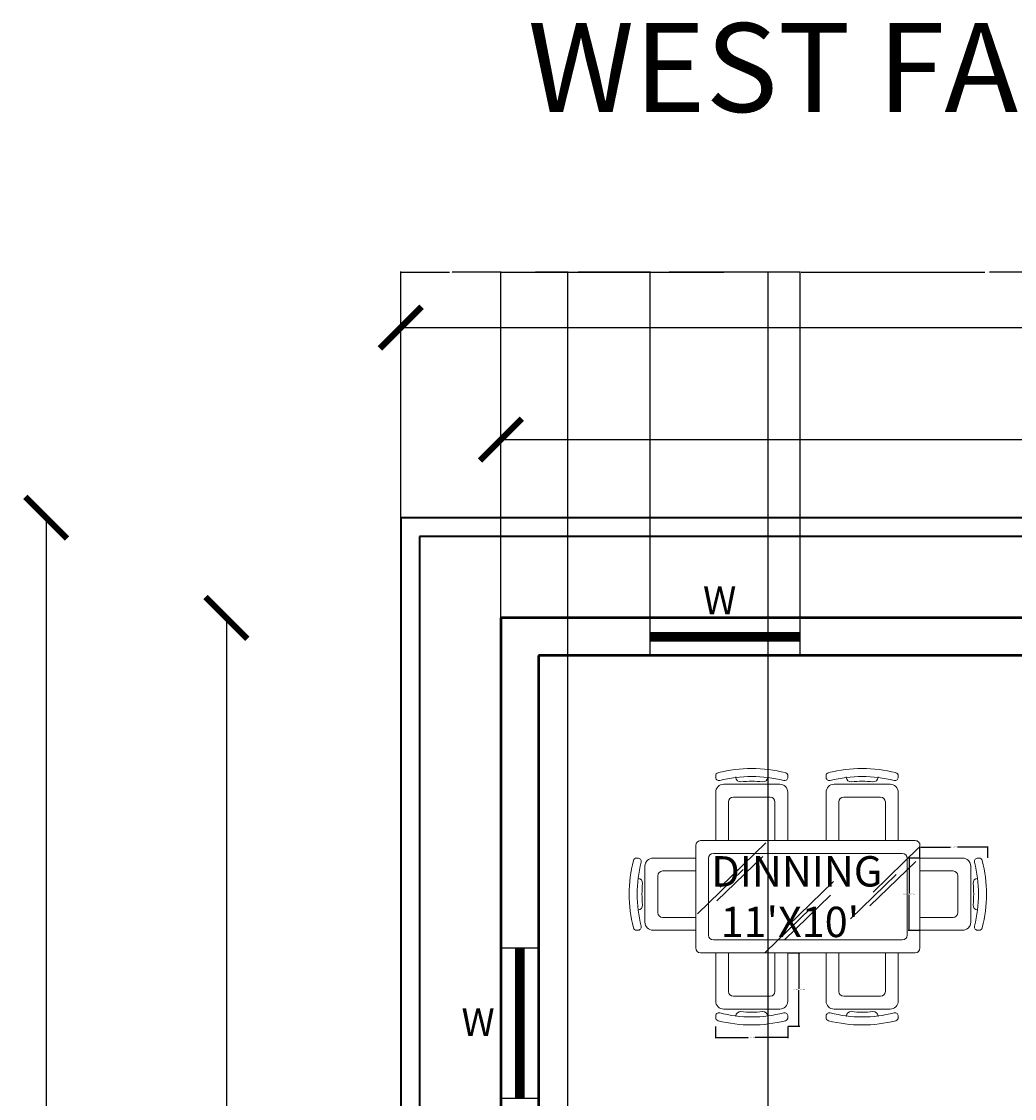
# Model space of a CAD drawing. Units: inches. Extents: x 338 to 1188, y -996 to 127.
# Tile 7 of 15: x 482 to 720, y -131 to 127. Entities that reach past the tile are written whole.
import ezdxf

# ---------------------------------------------------------------- set-up
doc = ezdxf.new("R2010")
doc.units = ezdxf.units.IN
doc.header["$MEASUREMENT"] = 0
for name, color, linetype, lineweight in [('A-ANNO-DIMS', 5, 'Continuous', 18), ('A-ANNO-TEXT', 7, 'Continuous', 18), ('A-ANNO-TITL', 7, 'Continuous', 35), ('A-AREA-IDEN', 8, 'Continuous', 18), ('A-GLAZ-PATT', 5, 'Continuous', 13), ('C-PROP', 1, 'Continuous', 35), ('wall', 1, 'Continuous', 50), ('win', 5, 'Continuous', 25)]:
    doc.layers.add(name, color=color, linetype=linetype, lineweight=lineweight)
doc.layers.add('furniture', color=50, linetype='Continuous', lineweight=13, transparency=0.8)
doc.styles.get("Standard").update_dxf_attribs({"font": 'arial.ttf'})
doc.dimstyles.get("Standard").update_dxf_attribs({"dimtxt": 0.18, "dimasz": 0.18, "dimexe": 0.18, "dimexo": 0.0625, "dimgap": 0.09, "dimtad": 0, "dimtih": 1, "dimtoh": 1, "dimdec": 1, "dimzin": 0, "dimdsep": 46, "dimlunit": 4, "dimtxsty": 'Standard', "dimcen": 0.09, "dimadec": 0, "dimazin": 0, "dimtfac": 1, "dimtdec": 1, "dimtofl": 0, "dimtmove": 0, "dimatfit": 3, "dimfxl": 1, "dimtolj": 1, "dimtzin": 0, "dimarcsym": 0})

# ---------------------------------------------------------------- blocks, each defined once
blk = doc.blocks.new('_ArchTick')
at = {"color": 0, "linetype": 'ByBlock', "const_width": 0.15}
blk.add_lwpolyline([(-0.5, -0.5), (0.5, 0.5)], dxfattribs=at)
blk = doc.blocks.new('*D4')
at = {"layer": 'A-ANNO-DIMS', "color": 0, "lineweight": -2, "transparency": 16777216}
for p, q in [((596.96, 26.99), (765.33, 26.99)), ((956.96, 26.99), (788.6, 26.99))]:
    blk.add_line(p, q, dxfattribs=at)
at = {"layer": 'Defpoints', "color": 0, "transparency": 16777216}
for p in [(956.96, 26.99), (596.96, -15.73), (956.96, -15.73)]:
    blk.add_point(p, dxfattribs=at)
at = {"layer": 'A-ANNO-DIMS', "color": 0, "lineweight": -2, "transparency": 16777216, "xscale": 10, "yscale": 10, "zscale": 10, "rotation": 180}
blk.add_blockref('_ArchTick', (596.96, 26.99), dxfattribs=at)
at = {"layer": 'A-ANNO-DIMS', "color": 0, "lineweight": -2, "transparency": 16777216, "xscale": 10, "yscale": 10, "zscale": 10}
blk.add_blockref('_ArchTick', (956.96, 26.99), dxfattribs=at)
at = {"layer": 'A-ANNO-DIMS', "color": 0, "transparency": 16777216, "insert": (776.96, 26.99), "char_height": 9, "attachment_point": 5}
blk.add_mtext("\\A1;30'", dxfattribs=at)
blk = doc.blocks.new('*D5')
at = {"layer": 'A-ANNO-DIMS', "color": 0, "lineweight": -2, "transparency": 16777216}
for p, q in [((572.96, 53.81), (765.33, 53.81)), ((980.96, 53.81), (788.6, 53.81))]:
    blk.add_line(p, q, dxfattribs=at)
at = {"layer": 'Defpoints', "color": 0, "transparency": 16777216}
for p in [(980.96, 53.81), (572.96, 8.27), (980.96, 8.27)]:
    blk.add_point(p, dxfattribs=at)
at = {"layer": 'A-ANNO-DIMS', "color": 0, "lineweight": -2, "transparency": 16777216, "xscale": 10, "yscale": 10, "zscale": 10, "rotation": 180}
blk.add_blockref('_ArchTick', (572.96, 53.81), dxfattribs=at)
at = {"layer": 'A-ANNO-DIMS', "color": 0, "lineweight": -2, "transparency": 16777216, "xscale": 10, "yscale": 10, "zscale": 10}
blk.add_blockref('_ArchTick', (980.96, 53.81), dxfattribs=at)
at = {"layer": 'A-ANNO-DIMS', "color": 0, "transparency": 16777216, "insert": (776.96, 53.81), "char_height": 9, "attachment_point": 5}
blk.add_mtext("\\A1;34'", dxfattribs=at)
blk = doc.blocks.new('*D6')
at = {"layer": 'A-ANNO-DIMS', "color": 0, "lineweight": -2, "transparency": 16777216}
for p, q in [((531.19, -15.73), (531.19, -304.1)), ((531.19, -615.73), (531.19, -327.37))]:
    blk.add_line(p, q, dxfattribs=at)
at = {"layer": 'Defpoints', "color": 0, "transparency": 16777216}
for p in [(596.96, -15.73), (531.19, -615.73), (596.96, -615.73)]:
    blk.add_point(p, dxfattribs=at)
at = {"layer": 'A-ANNO-DIMS', "color": 0, "lineweight": -2, "transparency": 16777216, "xscale": 10, "yscale": 10, "zscale": 10}
for p, rotation in [((531.19, -15.73), 90), ((531.19, -615.73), 270)]:
    blk.add_blockref('_ArchTick', p, dxfattribs=dict(at, rotation=rotation))
at = {"layer": 'A-ANNO-DIMS', "color": 0, "transparency": 16777216, "insert": (531.19, -315.73), "char_height": 9, "attachment_point": 5, "rotation": 90}
blk.add_mtext("\\A1;50'", dxfattribs=at)
blk = doc.blocks.new('*D7')
at = {"layer": 'A-ANNO-DIMS', "color": 0, "lineweight": -2, "transparency": 16777216}
for p, q in [((488.01, 8.27), (488.01, -388.07)), ((488.01, -807.73), (488.01, -411.39))]:
    blk.add_line(p, q, dxfattribs=at)
at = {"layer": 'Defpoints', "color": 0, "transparency": 16777216}
for p in [(572.96, 8.27), (488.01, -807.73), (572.96, -807.73)]:
    blk.add_point(p, dxfattribs=at)
at = {"layer": 'A-ANNO-DIMS', "color": 0, "lineweight": -2, "transparency": 16777216, "xscale": 10, "yscale": 10, "zscale": 10}
for p, rotation in [((488.01, 8.27), 90), ((488.01, -807.73), 270)]:
    blk.add_blockref('_ArchTick', p, dxfattribs=dict(at, rotation=rotation))
at = {"layer": 'A-ANNO-DIMS', "color": 0, "transparency": 16777216, "insert": (488.01, -399.73), "char_height": 9, "attachment_point": 5, "rotation": 90}
blk.add_mtext("\\A1;68'", dxfattribs=at)
blk = doc.blocks.new('CHAIR-DINING-SIDE')
for p, q in [((6.72, 13.5), (-6.72, 13.5)), ((-3.84, 15.13), (-3.84, 15.25)), ((3.84, 15.13), (3.84, 15.25)), ((-8.63, 11.76), (-8.63, 11.36)), ((-8.63, 11.58), (-8.63, 0)), ((4.41, 10.43), (-4.41, 10.43)), ((8.63, 11.36), (8.63, 11.76)), ((8.63, 0), (8.63, 11.58)), ((-5.56, 9.28), (-5.56, 0)), ((5.56, 0), (5.56, 9.28))]:
    blk.add_line(p, q)
for centre, radius, start, end in [((-7.87, 15.54), 0.768, 104.147, 185.9216), ((0, -15.67), 32.96, 75.853, 104.147), ((7.87, 15.54), 0.768, 354.0784, 75.853), ((-9.78, 15.34), 1.15, 354.0784, 5.9216), ((-7.87, 15.15), 0.768, 174.0784, 284.3214), ((-6.72, 11.58), 1.92, 90, 180), ((0, -15.67), 31.04, 75.6786, 104.3214), ((-2.69, 15.25), 1.15, 186.0281, 274.9654), ((0, -15.67), 29.89, 85.0346, 94.9654), ((2.69, 15.25), 1.15, 265.0346, 353.9719), ((6.72, 11.58), 1.92, 0, 90), ((7.87, 15.15), 0.768, 255.6786, 5.9216), ((9.78, 15.34), 1.15, 174.0784, 185.9216), ((-4.41, 9.28), 1.15, 90, 180), ((4.41, 9.28), 1.15, 0, 90)]:
    blk.add_arc(centre, radius, start, end)
blk = doc.blocks.new('CHAIR-DINING-END')
for p, q in [((-10.42, 8.63), (-10.02, 8.63)), ((-10.24, 8.63), (0, 8.63)), ((-12.16, -6.72), (-12.16, 6.72)), ((-7.94, 5.56), (0, 5.56)), ((-13.79, 3.84), (-13.91, 3.84)), ((-9.09, -4.41), (-9.09, 4.41)), ((-13.79, -3.84), (-13.91, -3.84)), ((0, -5.56), (-7.94, -5.56)), ((-10.02, -8.63), (-10.42, -8.63)), ((0, -8.63), (-10.24, -8.63))]:
    blk.add_line(p, q)
for centre, radius, start, end in [((17.01, 0), 32.96, 165.853, 194.147), ((-14.2, 7.87), 0.768, 84.0784, 165.853), ((-14.01, 9.78), 1.15, 264.0784, 275.9216), ((-13.81, 7.87), 0.768, 345.6786, 95.9216), ((-10.24, 6.72), 1.92, 90, 180), ((17.01, 0), 31.04, 165.6786, 194.3214), ((-7.94, 4.41), 1.15, 90, 180), ((-13.91, 2.69), 1.15, 355.0346, 83.9719), ((17.01, 0), 29.89, 175.0346, 184.9654), ((-13.91, -2.69), 1.15, 276.0281, 4.9654), ((-7.94, -4.41), 1.15, 180, 270), ((-13.81, -7.87), 0.768, 264.0784, 14.3214), ((-10.24, -6.72), 1.92, 180, 270), ((-14.2, -7.87), 0.768, 194.147, 275.9216), ((-14.01, -9.78), 1.15, 84.0784, 95.9216)]:
    blk.add_arc(centre, radius, start, end)
blk = doc.blocks.new('*D15')
at = {"layer": 'A-ANNO-DIMS', "color": 0, "lineweight": -2, "transparency": 16777216}
for p, q in [((665.79, -95.98), (668.55, -95.98)), ((668.37, -96.16), (668.37, -104.6)), ((668.37, -113.42), (668.37, -104.97)), ((665.79, -113.6), (668.55, -113.6))]:
    blk.add_line(p, q, dxfattribs=at)
at = {"layer": 'A-ANNO-DIMS', "color": 0, "transparency": 16777216}
for points in [[(668.34, -96.16), (668.4, -96.16), (668.37, -95.98)], [(668.34, -113.42), (668.4, -113.42), (668.37, -113.6)]]:
    blk.add_solid(points, dxfattribs=at)
at = {"layer": 'Defpoints', "color": 0, "transparency": 16777216}
for p in [(665.73, -95.98), (665.73, -113.6), (668.37, -113.6)]:
    blk.add_point(p, dxfattribs=at)
at = {"layer": 'A-ANNO-DIMS', "color": 0, "transparency": 16777216, "insert": (668.37, -104.79), "char_height": 0.18, "attachment_point": 5}
blk.add_mtext('\\A1;SIDE CHAIR 1\'-5 1/2" TYP.', dxfattribs=at)
blk = doc.blocks.new('*D16')
at = {"layer": 'A-ANNO-DIMS', "color": 0, "lineweight": -2, "transparency": 16777216}
for p, q in [((648.39, -113.66), (648.39, -116.42)), ((665.73, -113.66), (665.73, -116.42)), ((648.57, -116.24), (656.22, -116.24)), ((665.55, -116.24), (657.9, -116.24))]:
    blk.add_line(p, q, dxfattribs=at)
at = {"layer": 'A-ANNO-DIMS', "color": 0, "transparency": 16777216}
for points in [[(648.57, -116.21), (648.57, -116.27), (648.39, -116.24)], [(665.55, -116.21), (665.55, -116.27), (665.73, -116.24)]]:
    blk.add_solid(points, dxfattribs=at)
at = {"layer": 'Defpoints', "color": 0, "transparency": 16777216}
for p in [(648.39, -113.6), (665.73, -113.6), (648.39, -116.24)]:
    blk.add_point(p, dxfattribs=at)
at = {"layer": 'A-ANNO-DIMS', "color": 0, "transparency": 16777216, "insert": (657.06, -116.24), "char_height": 0.18, "attachment_point": 5}
blk.add_mtext('\\A1;1\'-5 1/2" TYP.', dxfattribs=at)
blk = doc.blocks.new('*D17')
at = {"layer": 'A-ANNO-DIMS', "color": 0, "lineweight": -2, "transparency": 16777216}
for p, q in [((697.3, -73.27), (694.58, -73.27)), ((694.76, -73.45), (694.76, -81.76)), ((694.76, -90.43), (694.76, -82.12)), ((697.3, -90.61), (694.58, -90.61))]:
    blk.add_line(p, q, dxfattribs=at)
at = {"layer": 'A-ANNO-DIMS', "color": 0, "transparency": 16777216}
for points in [[(694.73, -73.45), (694.79, -73.45), (694.76, -73.27)], [(694.73, -90.43), (694.79, -90.43), (694.76, -90.61)]]:
    blk.add_solid(points, dxfattribs=at)
at = {"layer": 'Defpoints', "color": 0, "transparency": 16777216}
for p in [(697.36, -73.27), (694.76, -90.61), (697.36, -90.61)]:
    blk.add_point(p, dxfattribs=at)
at = {"layer": 'A-ANNO-DIMS', "color": 0, "transparency": 16777216, "insert": (694.76, -81.94), "char_height": 0.18, "attachment_point": 5}
blk.add_mtext('\\A1;END CHAIR 1\'-5 1/2" TYP.', dxfattribs=at)
blk = doc.blocks.new('*D18')
at = {"layer": 'A-ANNO-DIMS', "color": 0, "lineweight": -2, "transparency": 16777216}
for p, q in [((697.36, -73.21), (697.36, -70.49)), ((697.54, -70.67), (704.67, -70.67)), ((713.47, -70.67), (706.34, -70.67)), ((713.65, -73.21), (713.65, -70.49))]:
    blk.add_line(p, q, dxfattribs=at)
at = {"layer": 'A-ANNO-DIMS', "color": 0, "transparency": 16777216}
for points in [[(697.54, -70.64), (697.54, -70.7), (697.36, -70.67)], [(713.47, -70.64), (713.47, -70.7), (713.65, -70.67)]]:
    blk.add_solid(points, dxfattribs=at)
at = {"layer": 'Defpoints', "color": 0, "transparency": 16777216}
for p in [(697.36, -70.67), (697.36, -73.27), (713.65, -73.27)]:
    blk.add_point(p, dxfattribs=at)
at = {"layer": 'A-ANNO-DIMS', "color": 0, "transparency": 16777216, "insert": (705.51, -70.67), "char_height": 0.18, "attachment_point": 5}
blk.add_mtext('\\A1;1\'-4 1/2" TYP.', dxfattribs=at)
blk = doc.blocks.new('*D24')
at = {"layer": 'A-ANNO-DIMS', "color": 0, "lineweight": -2, "transparency": 16777216}
for p, q in [((572.96, 8.33), (572.96, 67.25)), ((596.96, -15.67), (596.96, 67.25)), ((573.14, 67.07), (584.63, 67.07)), ((596.78, 67.07), (585.29, 67.07))]:
    blk.add_line(p, q, dxfattribs=at)
at = {"layer": 'A-ANNO-DIMS', "color": 0, "transparency": 16777216}
for points in [[(573.14, 67.1), (573.14, 67.04), (572.96, 67.07)], [(596.78, 67.1), (596.78, 67.04), (596.96, 67.07)]]:
    blk.add_solid(points, dxfattribs=at)
at = {"layer": 'Defpoints', "color": 0, "transparency": 16777216}
for p in [(596.96, 67.07), (572.96, 8.27), (596.96, -15.73)]:
    blk.add_point(p, dxfattribs=at)
at = {"layer": 'A-ANNO-DIMS', "color": 0, "transparency": 16777216, "insert": (584.96, 67.07), "char_height": 0.18, "attachment_point": 5}
blk.add_mtext('\\A1;2\'-0"', dxfattribs=at)
blk = doc.blocks.new('*D33')
at = {"layer": 'A-ANNO-DIMS', "color": 0, "lineweight": -2, "transparency": 16777216}
for p, q in [((632.69, -15.67), (632.69, 67.25)), ((668.69, -15.67), (668.69, 67.25)), ((632.87, 67.07), (650.37, 67.07)), ((668.51, 67.07), (651.02, 67.07))]:
    blk.add_line(p, q, dxfattribs=at)
at = {"layer": 'A-ANNO-DIMS', "color": 0, "transparency": 16777216}
for points in [[(632.87, 67.1), (632.87, 67.04), (632.69, 67.07)], [(668.51, 67.1), (668.51, 67.04), (668.69, 67.07)]]:
    blk.add_solid(points, dxfattribs=at)
at = {"layer": 'Defpoints', "color": 0, "transparency": 16777216}
for p in [(668.69, 67.07), (632.69, -15.73), (668.69, -15.73)]:
    blk.add_point(p, dxfattribs=at)
at = {"layer": 'A-ANNO-DIMS', "color": 0, "transparency": 16777216, "insert": (650.69, 67.07), "char_height": 0.18, "attachment_point": 5}
blk.add_mtext('\\A1;3\'-0"', dxfattribs=at)
blk = doc.blocks.new('*D34')
at = {"layer": 'A-ANNO-DIMS', "color": 0, "lineweight": -2, "transparency": 16777216}
for p, q in [((612.96, -615.67), (612.96, 67.25)), ((660.96, -615.67), (660.96, 67.25)), ((613.14, 67.07), (636.63, 67.07)), ((660.78, 67.07), (637.3, 67.07))]:
    blk.add_line(p, q, dxfattribs=at)
at = {"layer": 'A-ANNO-DIMS', "color": 0, "transparency": 16777216}
for points in [[(613.14, 67.1), (613.14, 67.04), (612.96, 67.07)], [(660.78, 67.1), (660.78, 67.04), (660.96, 67.07)]]:
    blk.add_solid(points, dxfattribs=at)
at = {"layer": 'Defpoints', "color": 0, "transparency": 16777216}
for p in [(660.96, 67.07), (612.96, -615.73), (660.96, -615.73)]:
    blk.add_point(p, dxfattribs=at)
at = {"layer": 'A-ANNO-DIMS', "color": 0, "transparency": 16777216, "insert": (636.96, 67.07), "char_height": 0.18, "attachment_point": 5}
blk.add_mtext('\\A1;4\'-0"', dxfattribs=at)
blk = doc.blocks.new('*D48')
at = {"layer": 'A-ANNO-DIMS', "color": 0, "lineweight": -2, "transparency": 16777216}
for p, q in [((596.96, -615.67), (596.96, 67.25)), ((612.96, -615.67), (612.96, 67.25)), ((597.14, 67.07), (604.64, 67.07)), ((612.78, 67.07), (605.28, 67.07))]:
    blk.add_line(p, q, dxfattribs=at)
at = {"layer": 'A-ANNO-DIMS', "color": 0, "transparency": 16777216}
for points in [[(597.14, 67.1), (597.14, 67.04), (596.96, 67.07)], [(612.78, 67.1), (612.78, 67.04), (612.96, 67.07)]]:
    blk.add_solid(points, dxfattribs=at)
at = {"layer": 'Defpoints', "color": 0, "transparency": 16777216}
for p in [(612.96, 67.07), (596.96, -615.73), (612.96, -615.73)]:
    blk.add_point(p, dxfattribs=at)
at = {"layer": 'A-ANNO-DIMS', "color": 0, "transparency": 16777216, "insert": (604.96, 67.07), "char_height": 0.18, "attachment_point": 5}
blk.add_mtext('\\A1;1\'-4"', dxfattribs=at)
blk = doc.blocks.new('*D49')
at = {"layer": 'A-ANNO-DIMS', "color": 0, "lineweight": -2, "transparency": 16777216}
for p, q in [((596.96, -15.67), (596.96, 67.25)), ((632.69, -15.67), (632.69, 67.25)), ((597.14, 67.07), (614.22, 67.07)), ((632.51, 67.07), (615.44, 67.07))]:
    blk.add_line(p, q, dxfattribs=at)
at = {"layer": 'A-ANNO-DIMS', "color": 0, "transparency": 16777216}
for points in [[(597.14, 67.1), (597.14, 67.04), (596.96, 67.07)], [(632.51, 67.1), (632.51, 67.04), (632.69, 67.07)]]:
    blk.add_solid(points, dxfattribs=at)
at = {"layer": 'Defpoints', "color": 0, "transparency": 16777216}
for p in [(632.69, 67.07), (596.96, -15.73), (632.69, -15.73)]:
    blk.add_point(p, dxfattribs=at)
at = {"layer": 'A-ANNO-DIMS', "color": 0, "transparency": 16777216, "insert": (614.83, 67.07), "char_height": 0.18, "attachment_point": 5}
blk.add_mtext('\\A1;2\'-11 1/2"', dxfattribs=at)
blk = doc.blocks.new('*D50')
at = {"layer": 'A-ANNO-DIMS', "color": 0, "lineweight": -2, "transparency": 16777216}
for p, q in [((668.69, -15.67), (668.69, 67.25)), ((758.21, -15.67), (758.21, 67.25)), ((668.87, 67.07), (712.91, 67.07)), ((758.03, 67.07), (713.99, 67.07))]:
    blk.add_line(p, q, dxfattribs=at)
at = {"layer": 'A-ANNO-DIMS', "color": 0, "transparency": 16777216}
for points in [[(668.87, 67.1), (668.87, 67.04), (668.69, 67.07)], [(758.03, 67.1), (758.03, 67.04), (758.21, 67.07)]]:
    blk.add_solid(points, dxfattribs=at)
at = {"layer": 'Defpoints', "color": 0, "transparency": 16777216}
for p in [(758.21, 67.07), (668.69, -15.73), (758.21, -15.73)]:
    blk.add_point(p, dxfattribs=at)
at = {"layer": 'A-ANNO-DIMS', "color": 0, "transparency": 16777216, "insert": (713.45, 67.07), "char_height": 0.18, "attachment_point": 5}
blk.add_mtext('\\A1;7\'-5 1/2"', dxfattribs=at)

msp = doc.modelspace()

# ---------------------------------------------------------------- hatches: boundary and pattern name
at = {"layer": 'A-GLAZ-PATT'}
h = msp.add_hatch(dxfattribs=at)
h.set_pattern_fill('ANSI31', color=256)
h.paths.add_polyline_path([(953.46, -405.07), (951.46, -405.07), (951.46, -429.07), (953.46, -429.07)])
h.paths.add_polyline_path([(953.46, -485.22), (951.46, -485.22), (951.46, -521.22), (953.46, -521.22)])
h.paths.add_polyline_path([(794.21, -19.23), (758.21, -19.23), (758.21, -21.23), (794.21, -21.23)])
h.paths.add_polyline_path([(668.69, -19.23), (632.69, -19.23), (632.69, -21.23), (668.69, -21.23)])
h.paths.add_polyline_path([(602.46, -94.89), (600.46, -94.89), (600.46, -130.89), (602.46, -130.89)])
h.paths.add_polyline_path([(602.46, -243.73), (600.46, -243.73), (600.46, -315.73), (602.46, -315.73)])

# ---------------------------------------------------------------- linework, layer by layer
at = {"layer": 'C-PROP'}
for p, q in [((572.96, 8.27), (572.96, -807.73)), ((980.96, 8.27), (572.96, 8.27)), ((976.46, 3.77), (577.46, 3.77)), ((577.46, 3.77), (577.46, -803.23))]:
    msp.add_line(p, q, dxfattribs=at)
at = {"layer": 'furniture'}
for p, q in [((696.21, -69.11), (644.79, -69.11)), ((660.46, -69.61), (649.48, -80.24)), ((643.64, -70.26), (643.64, -94.83)), ((693.14, -72.18), (647.86, -72.18)), ((697.12, -70.79), (686.14, -81.42)), ((697.36, -94.83), (697.36, -70.26)), ((646.71, -73.33), (646.71, -91.76)), ((659.7, -72.92), (648.72, -83.56)), ((696.35, -74.11), (685.37, -84.74)), ((694.29, -91.76), (694.29, -73.33)), ((655.02, -76.01), (644.04, -86.65)), ((691.68, -77.2), (680.7, -87.83)), ((676.68, -78.89), (665.7, -89.53)), ((675.91, -82.21), (664.93, -92.84)), ((671.24, -85.3), (660.26, -95.93)), ((647.86, -92.91), (693.14, -92.91)), ((644.79, -95.98), (696.21, -95.98))]:
    msp.add_line(p, q, dxfattribs=at)
for centre, radius, start, end in [((644.79, -70.26), 1.15, 90, 180), ((696.27, -70.21), 1.1, 357.166, 92.834), ((647.86, -73.33), 1.15, 90, 180), ((693.14, -73.33), 1.15, 0, 90), ((647.86, -91.76), 1.15, 180, 270), ((693.14, -91.76), 1.15, 270, 0), ((644.79, -94.83), 1.15, 180, 270), ((696.21, -94.83), 1.15, 270, 0)]:
    msp.add_arc(centre, radius, start, end, dxfattribs=at)
at = {"layer": 'wall'}
for p, q in [((596.96, -15.73), (596.96, -615.73)), ((956.96, -15.73), (596.96, -15.73)), ((605.96, -24.73), (605.96, -144.73)), ((605.96, -24.73), (605.96, -144.73)), ((737.96, -24.73), (605.96, -24.73))]:
    msp.add_line(p, q, dxfattribs=at)
at = {"layer": 'win'}
for p, q in [((632.69, -24.73), (632.69, -15.73)), ((668.69, -24.73), (668.69, -15.73)), ((632.69, -19.23), (668.69, -19.23)), ((632.69, -21.23), (668.69, -21.23)), ((605.96, -94.89), (596.96, -94.89)), ((600.46, -94.89), (600.46, -130.89)), ((602.46, -94.89), (602.46, -130.89)), ((605.96, -130.89), (596.96, -130.89))]:
    msp.add_line(p, q, dxfattribs=at)

# ---------------------------------------------------------------- block references
at = {"layer": 'furniture'}
for name, p in [('CHAIR-DINING-SIDE', (657.06, -69.11)), ('CHAIR-DINING-SIDE', (683.51, -69.11)), ('CHAIR-DINING-END', (643.64, -81.94))]:
    msp.add_blockref(name, p, dxfattribs=at)
at = {"layer": 'furniture', "rotation": 180}
for name, p in [('CHAIR-DINING-END', (697.36, -81.94)), ('CHAIR-DINING-SIDE', (657.06, -95.98)), ('CHAIR-DINING-SIDE', (683.51, -95.98))]:
    msp.add_blockref(name, p, dxfattribs=at)

# ---------------------------------------------------------------- texts
at = {"layer": 'A-ANNO-TEXT'}
for p in [(645.39, -14.86), (587.51, -115.91)]:
    msp.add_text('W', height=6.65, dxfattribs=at).set_placement(p)
at = {"layer": 'A-ANNO-TITL', "insert": (603.41, 126.77), "char_height": 21.2807, "attachment_point": 1}
msp.add_mtext_dynamic_manual_height_columns('WEST FACING HOUSE', width=345.7385, gutter_width=3.55, heights=[0], dxfattribs=at)
at = {"layer": 'A-AREA-IDEN', "insert": (638.48, -72.83), "char_height": 7.2703, "attachment_point": 1}
msp.add_mtext_dynamic_manual_height_columns("    DINNING\\P     11'X10'", width=53.3957, gutter_width=1, heights=[0], dxfattribs=at)

# ---------------------------------------------------------------- dimensions: what is measured, and where the dimension line sits
at = {"layer": 'A-ANNO-DIMS'}
for base, p1, p2, override, picture, middle in [((596.96, 67.07), (572.96, 8.27), (596.96, -15.73), {"dimdec": 1, "dimlfac": 1, "dimrnd": 0, "dimzin": 1, "dimdsep": 46, "dimlunit": 4, "dimfrac": 2}, '*D24', (584.96, 67.07)), ((632.69, 67.07), (596.96, -15.73), (632.69, -15.73), {"dimdec": 1, "dimlfac": 1, "dimrnd": 0, "dimzin": 1, "dimdsep": 46, "dimlunit": 4, "dimfrac": 2}, '*D49', (614.83, 67.07)), ((612.96, 67.07), (596.96, -615.73), (612.96, -615.73), {"dimdec": 1, "dimlfac": 1, "dimrnd": 0, "dimzin": 1, "dimdsep": 46, "dimlunit": 4, "dimfrac": 2}, '*D48', (604.96, 67.07)), ((660.96, 67.07), (612.96, -615.73), (660.96, -615.73), {"dimdec": 1, "dimlfac": 1, "dimrnd": 0, "dimzin": 1, "dimdsep": 46, "dimlunit": 4, "dimfrac": 2}, '*D34', (636.96, 67.07)), ((668.69, 67.07), (632.69, -15.73), (668.69, -15.73), {"dimdec": 1, "dimlfac": 1, "dimrnd": 0, "dimzin": 1, "dimdsep": 46, "dimlunit": 4, "dimfrac": 2}, '*D33', (650.69, 67.07)), ((758.21, 67.07), (668.69, -15.73), (758.21, -15.73), {"dimdec": 1, "dimlfac": 1, "dimrnd": 0, "dimzin": 1, "dimdsep": 46, "dimlunit": 4, "dimfrac": 2}, '*D50', (713.45, 67.07)), ((980.96, 53.81), (572.96, 8.27), (980.96, 8.27), {"dimtxt": 9, "dimasz": 10, "dimgap": 4, "dimblk1": 'ArchTick', "dimblk2": 'ArchTick', "dimsah": 1, "dimse1": 1, "dimse2": 1, "dimclrd": 0, "dimclre": 0, "dimclrt": 0}, '*D5', (776.96, 53.81)), ((956.96, 26.99), (596.96, -15.73), (956.96, -15.73), {"dimtxt": 9, "dimasz": 10, "dimgap": 4, "dimblk1": 'ArchTick', "dimblk2": 'ArchTick', "dimsah": 1, "dimse1": 1, "dimse2": 1, "dimclrd": 0, "dimclre": 0, "dimclrt": 0}, '*D4', (776.96, 26.99))]:
    dim = msp.add_linear_dim(base=base, p1=p1, p2=p2, dimstyle='Standard', override=override, dxfattribs=at)
    dim.commit()
    dim.dimension.update_dxf_attribs({"geometry": picture, "text_midpoint": middle})
for base, p1, p2, override, picture, middle in [((488.01, -807.73), (572.96, 8.27), (572.96, -807.73), {"dimtxt": 9, "dimasz": 10, "dimgap": 4, "dimtad": 0, "dimtih": 0, "dimblk1": 'ArchTick', "dimblk2": 'ArchTick', "dimsah": 1, "dimse1": 1, "dimse2": 1, "dimclrd": 0, "dimclre": 0, "dimclrt": 0}, '*D7', (488.01, -399.73)), ((531.19, -615.73), (596.96, -15.73), (596.96, -615.73), {"dimtxt": 9, "dimasz": 10, "dimgap": 4, "dimtih": 0, "dimblk1": 'ArchTick', "dimblk2": 'ArchTick', "dimsah": 1, "dimse1": 1, "dimse2": 1, "dimclrd": 0, "dimclre": 0, "dimclrt": 0}, '*D6', (531.19, -315.73))]:
    dim = msp.add_linear_dim(base=base, p1=p1, p2=p2, angle=90, dimstyle='Standard', override=override, dxfattribs=at)
    dim.commit()
    dim.dimension.update_dxf_attribs({"geometry": picture, "text_midpoint": middle})
for base, p1, p2, angle, text, picture, middle in [((697.36, -70.67), (713.65, -73.27), (697.36, -73.27), 180, '<> TYP.', '*D18', (705.51, -70.67)), ((694.76, -90.61), (697.36, -73.27), (697.36, -90.61), 270, 'END CHAIR <> TYP.', '*D17', (694.76, -81.94)), ((668.37, -113.6), (665.73, -95.98), (665.73, -113.6), 270, 'SIDE CHAIR <> TYP.', '*D15', (668.37, -104.79)), ((648.39, -116.24), (665.73, -113.6), (648.39, -113.6), 180, '<> TYP.', '*D16', (657.06, -116.24))]:
    dim = msp.add_linear_dim(base=base, p1=p1, p2=p2, angle=angle, text=text, dimstyle='Standard', override={"dimdec": 1, "dimlfac": 1, "dimrnd": 0, "dimzin": 1, "dimdsep": 46, "dimlunit": 4, "dimfrac": 2}, dxfattribs=at)
    dim.commit()
    dim.dimension.update_dxf_attribs({"geometry": picture, "text_midpoint": middle})

doc.saveas('drawing.dxf')
